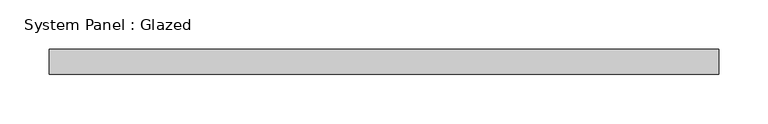
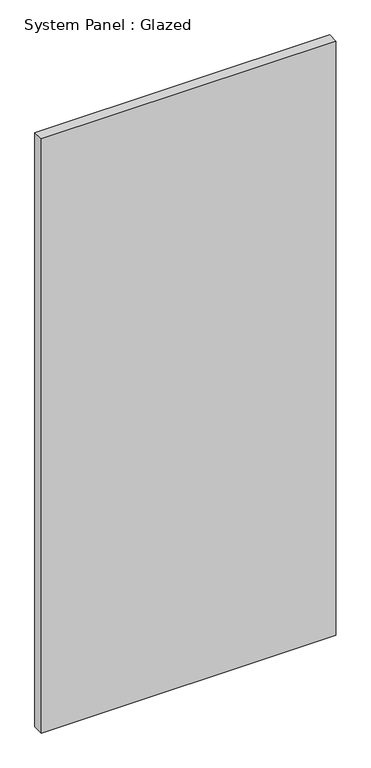
"""IFC4 building model written with IfcOpenShell, lengths in millimetres: plate geometry, System Panel : Glazed."""

from ifc_helpers import new_model, si_unit, origin, origin_with_axes, place, context, project, spatial, polyline, outline, extrude, source, transform, mapped, element, save


def system_panel_glazed_6ec13f64(model_context):
    return source(origin(), model_context, "Body", "SweptSolid", [
        extrude(outline(polyline([(339.725, 19.05), (-339.725, 19.05), (-339.725, 44.45), (339.725, 44.45), (339.725, 19.05)])), origin_with_axes(), (0.0, 0.0, 1.0), 1448.4674874),
    ])


if __name__ == "__main__":
    model = new_model("IFC4")
    model_context = context("Model", 3, world=origin())
    ifc_project = project(units=[si_unit("LENGTHUNIT", "METRE", prefix="MILLI")], contexts=[model_context])
    site = spatial("IfcSite", under=ifc_project)
    building = spatial("IfcBuilding", under=site)
    placement = place(None, origin())
    system_panel_glazed_shape = system_panel_glazed_6ec13f64(model_context)
    element("IfcPlate", 1, ObjectType="System Panel : Glazed", at=placement, inside=building, context=model_context, shape_type="MappedRepresentation", body=[
        mapped(system_panel_glazed_shape, transform((0.0, 0.0, 0.0), x_axis=(1.0, 0.0, 0.0), y_axis=(0.0, 1.0, 0.0), z_axis=(0.0, 0.0, 1.0))),
    ])
    save(model, "model.ifc")

# Revit data of these elements
# Type "System Panel : Glazed"
#   Construction Type Id = "GSP4R"
#   Analytic Construction = "1/8 in Pilkington single glazing"
#   Visual Light Transmittance = 0.9
#   Solar Heat Gain Coefficient = 0.86
#   Heat Transfer Coefficient (U) = 1.18115 BTU/(h·ft²·°F)
#   Define Thermal Properties by = 1
# Element 1 (IfcPlate, "System Panel : Glazed")
#   Materials on its faces: "Glass"
# Materials
#   "Glass": class "Glass", colour RGB 0 128 192, transparency 0.75, Description = "Soda Lime Glass", Cost = 0
